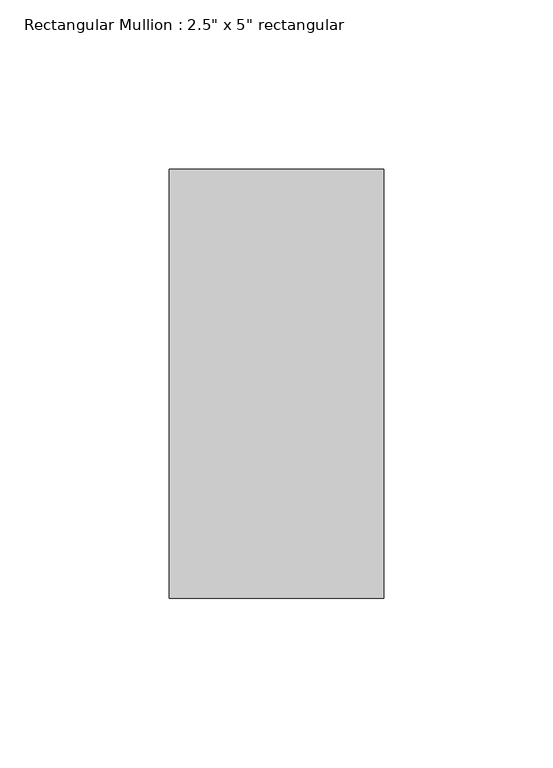
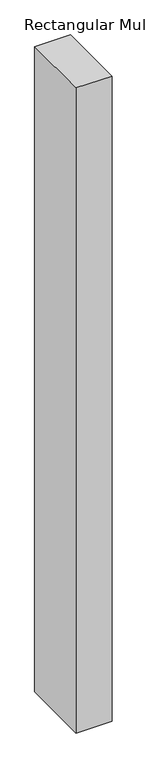
"""IFC4 building model written with IfcOpenShell, lengths in millimetres: member geometry."""

from ifc_helpers import new_model, si_unit, frame, origin, place, context, project, spatial, polyline, outline, extrude, source, transform, mapped, element, save


def member_91edd790(model_context):
    return source(origin(), model_context, "Body", "SweptSolid", [
        extrude(outline(polyline([(0.0, 63.5), (0.0, -63.5), (-63.5, -63.5), (-63.5, 63.5), (0.0, 63.5)])), frame((0.0, 0.0, -1206.4999998), z_axis=(0.0, 0.0, 1.0), x_axis=(1.0, 0.0, 0.0)), (0.0, 0.0, 1.0), 1206.4999998),
    ])


if __name__ == "__main__":
    model = new_model("IFC4")
    model_context = context("Model", 3, world=origin())
    ifc_project = project(units=[si_unit("LENGTHUNIT", "METRE", prefix="MILLI")], contexts=[model_context])
    site = spatial("IfcSite", under=ifc_project)
    building = spatial("IfcBuilding", under=site)
    placement = place(None, origin())
    member_shape = member_91edd790(model_context)
    element("IfcMember", 1, ObjectType="Rectangular Mullion : 2.5\" x 5\" rectangular", at=placement, inside=building, context=model_context, shape_type="MappedRepresentation", body=[
        mapped(member_shape, transform((0.0, 0.0, 0.0), x_axis=(1.0, 0.0, 0.0), y_axis=(0.0, 1.0, 0.0), z_axis=(0.0, 0.0, 1.0))),
    ])
    save(model, "model.ifc")

# Revit data of these elements
# Type "Rectangular Mullion : 2.5\" x 5\" rectangular"
#   built-in parameter 1007304 = 0.416667 (stored number, unit not read)
#   built-in parameter 1007301 = 0.104167 (stored number, unit not read)
#   built-in parameter 1007300 = 0.104167 (stored number, unit not read)
# Element 1 (IfcMember, "Rectangular Mullion : 2.5\" x 5\" rectangular")
#   Materials on its faces: "WINDOW FRAMING"
# Materials
#   "WINDOW FRAMING": class "Generic", colour RGB 120 120 120, transparency 0, Cost = 0
